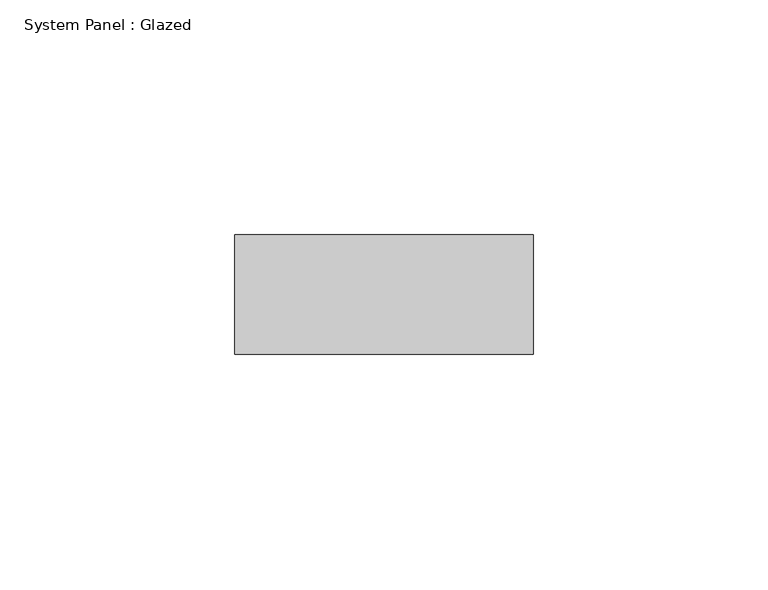
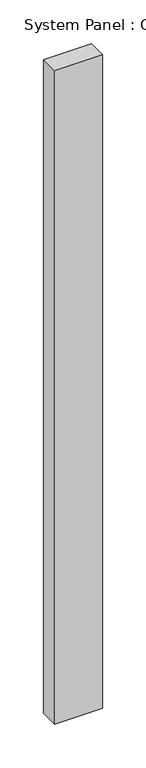
"""IFC4 building model written with IfcOpenShell, lengths in millimetres: plate geometry, System Panel : Glazed."""

from ifc_helpers import new_model, si_unit, origin, origin_with_axes, place, context, project, spatial, polyline, outline, extrude, source, transform, mapped, element, save


def system_panel_glazed_836907cd(model_context):
    return source(origin(), model_context, "Body", "SweptSolid", [
        extrude(outline(polyline([(31.75, 19.05), (-31.75, 19.05), (-31.75, 44.45), (31.75, 44.45), (31.75, 19.05)])), origin_with_axes(), (0.0, 0.0, 1.0), 914.4),
    ])


if __name__ == "__main__":
    model = new_model("IFC4")
    model_context = context("Model", 3, world=origin())
    ifc_project = project(units=[si_unit("LENGTHUNIT", "METRE", prefix="MILLI")], contexts=[model_context])
    site = spatial("IfcSite", under=ifc_project)
    building = spatial("IfcBuilding", under=site)
    placement = place(None, origin())
    system_panel_glazed_shape = system_panel_glazed_836907cd(model_context)
    element("IfcPlate", 1, ObjectType="System Panel : Glazed", at=placement, inside=building, context=model_context, shape_type="MappedRepresentation", body=[
        mapped(system_panel_glazed_shape, transform((0.0, 0.0, 0.0), x_axis=(1.0, 0.0, 0.0), y_axis=(0.0, 1.0, 0.0), z_axis=(0.0, 0.0, 1.0))),
    ])
    save(model, "model.ifc")

# Revit data of these elements
# Type "System Panel : Glazed"
#   Construction Type Id = "GSP4R"
#   Analytic Construction = "1/8 in Pilkington single glazing"
#   Visual Light Transmittance = 0.9
#   Solar Heat Gain Coefficient = 0.86
#   Heat Transfer Coefficient (U) = 6.7069 W/(m²·K)
# Element 1 (IfcPlate, "System Panel : Glazed")
#   Materials on its faces: "Glass"
# Materials
#   "Glass": class "Glass", colour RGB 0 128 192, transparency 0.75, Description = "Soda Lime Glass", Cost = 0
